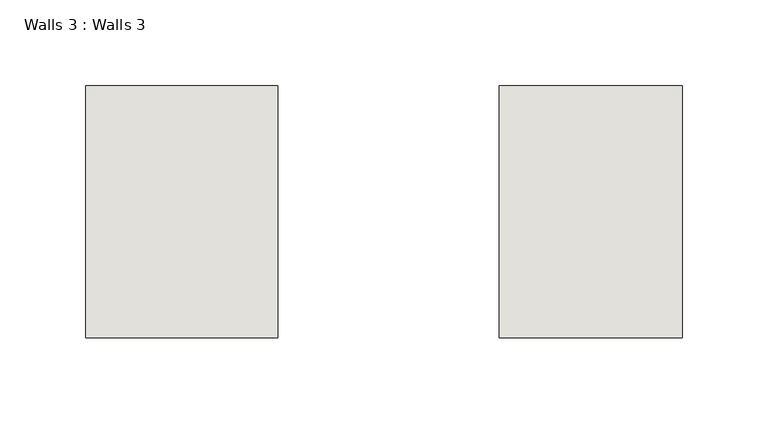
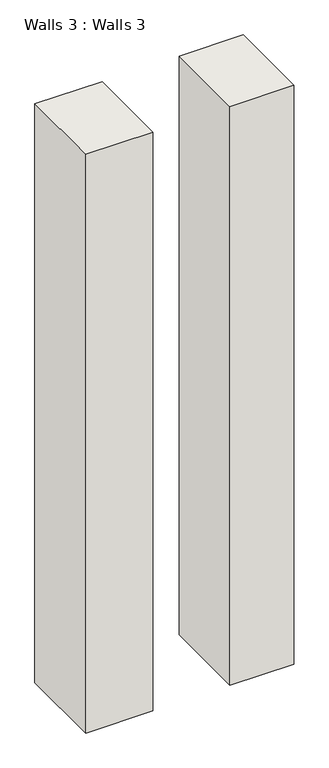
"""IFC4 building model written with IfcOpenShell, lengths in millimetres: wall geometry, Walls 3 : Walls 3."""

from ifc_helpers import new_model, si_unit, frame, origin, place, context, project, spatial, polyline, outline, extrude, source, transform, mapped, element, save


def walls_3_walls_3_33d2e255(model_context):
    return source(origin(), model_context, "Body", "SweptSolid", [
        extrude(outline(polyline([(-8099.5132571, -1530.0500552), (-8211.3408017, -1530.0500552), (-8211.3408017, -1383.4895946), (-8099.5132571, -1383.4895946), (-8099.5132571, -1530.0500552)])), frame((0.0, 0.0, 7620.0), z_axis=(0.0, 0.0, 1.0), x_axis=(1.0, 0.0, 0.0)), (0.0, 0.0, 1.0), 1019.9265532),
        extrude(outline(polyline([(-7864.267961, -1530.0500552), (-7970.830897, -1530.0500552), (-7970.830897, -1383.4895946), (-7864.267961, -1383.4895946), (-7864.267961, -1530.0500552)])), frame((0.0, 0.0, 7620.0), z_axis=(0.0, 0.0, 1.0), x_axis=(1.0, 0.0, 0.0)), (0.0, 0.0, 1.0), 1019.9265532),
    ])


if __name__ == "__main__":
    model = new_model("IFC4")
    model_context = context("Model", 3, world=origin())
    ifc_project = project(units=[si_unit("LENGTHUNIT", "METRE", prefix="MILLI")], contexts=[model_context])
    site = spatial("IfcSite", under=ifc_project)
    building = spatial("IfcBuilding", under=site)
    placement = place(None, origin())
    walls_3_walls_3_shape = walls_3_walls_3_33d2e255(model_context)
    element("IfcWall", 1, ObjectType="Walls 3 : Walls 3", at=placement, inside=building, context=model_context, shape_type="MappedRepresentation", body=[
        mapped(walls_3_walls_3_shape, transform((0.0, 0.0, 0.0), x_axis=(1.0, 0.0, 0.0), y_axis=(0.0, 1.0, 0.0), z_axis=(0.0, 0.0, 1.0))),
    ])
    save(model, "model.ifc")

# Revit data of these elements
# Element 1 (IfcWall, "Walls 3 : Walls 3")
#   Materials on its faces: "Default Wall"
# Materials
#   "Default Wall": colour RGB 128 128 128, transparency 0
